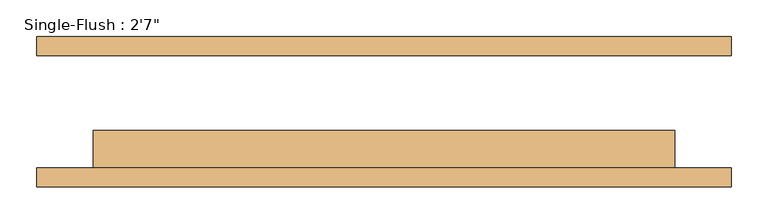
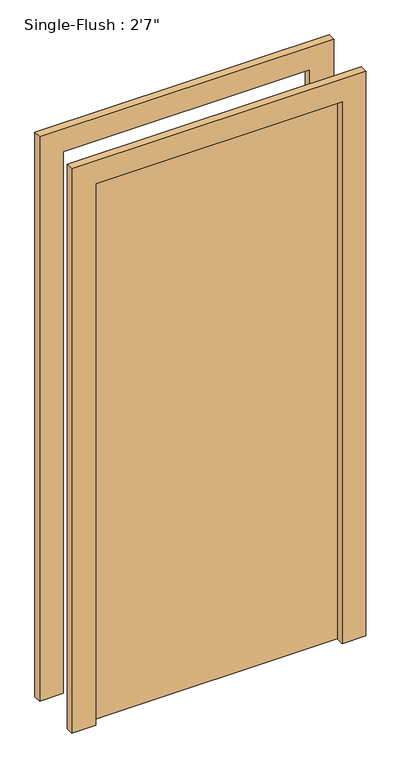
"""IFC4 building model written with IfcOpenShell, lengths in millimetres: door geometry."""

from ifc_helpers import new_model, si_unit, frame, origin, origin_with_axes, place, context, project, spatial, polyline, outline, extrude, source, transform, mapped, element, save


def door_ee35e093(model_context):
    return source(origin(), model_context, "Body", "SweptSolid", [
        extrude(outline(polyline([(1905.0, -469.9), (0.0, -469.9), (0.0, -393.7), (1828.8, -393.7), (1828.8, 393.7), (0.0, 393.7), (0.0, 469.9), (1905.0, 469.9), (1905.0, -469.9)])), frame((0.0, -101.6, 0.0), z_axis=(0.0, 1.0, 0.0), x_axis=(0.0, 0.0, 1.0)), (0.0, 0.0, 1.0), 25.4),
        extrude(outline(polyline([(1905.0, 469.9), (1905.0, -469.9), (0.0, -469.9), (0.0, -393.7), (1828.8, -393.7), (1828.8, 393.7), (0.0, 393.7), (0.0, 469.9), (1905.0, 469.9)])), frame((0.0, 76.2, 0.0), z_axis=(0.0, 1.0, 0.0), x_axis=(0.0, 0.0, 1.0)), (0.0, 0.0, 1.0), 25.4),
        extrude(outline(polyline([(393.7, -25.4), (393.7, -76.2), (-393.7, -76.2), (-393.7, -25.4), (393.7, -25.4)])), origin_with_axes(), (0.0, 0.0, 1.0), 1828.8),
    ])


if __name__ == "__main__":
    model = new_model("IFC4")
    model_context = context("Model", 3, world=origin())
    ifc_project = project(units=[si_unit("LENGTHUNIT", "METRE", prefix="MILLI")], contexts=[model_context])
    site = spatial("IfcSite", under=ifc_project)
    building = spatial("IfcBuilding", under=site)
    placement = place(None, origin())
    door_shape = door_ee35e093(model_context)
    element("IfcDoor", 1, ObjectType="Single-Flush : 2'7\"", at=placement, inside=building, context=model_context, shape_type="MappedRepresentation", body=[
        mapped(door_shape, transform((0.0, 0.0, 0.0), x_axis=(1.0, 0.0, 0.0), y_axis=(0.0, 1.0, 0.0), z_axis=(0.0, 0.0, 1.0))),
    ])
    save(model, "model.ifc")

# Revit data of these elements
# Type "Single-Flush : 2'7\""
#   Type Mark = "12"
#   Construction Type Id = "MDOOR"
#   Assembly Code = "C1020"
#   Analytic Construction = "Metal"
#   Thickness = 0' - 2"
#   Heat Transfer Coefficient (U) = 0.651978 BTU/(h·ft²·°F)
#   Height = 6' - 0"
#   Trim Projection Ext = 0' - 1"
#   Trim Projection Int = 0' - 1"
#   Trim Width = 0' - 3"
#   Width = 2' - 7"
#   Define Thermal Properties by = 1
#   Door Material = Door - Panel
#   Frame Material = Door - Frame
#   Visual Light Transmittance = 0
#   Solar Heat Gain Coefficient = 0
#   Function = (empty or 0)
#   Wall Closure = (empty or 0)
# Element 1 (IfcDoor, "Single-Flush : 2'7\"")
#   Materials on its faces: "Door - Frame", "Door - Panel"
# Materials
#   "Door - Panel": class "Wood", colour RGB 210 159 95, transparency 0, Cost = 0
#   "Door - Frame": colour RGB 118 70 51, transparency 0, Cost = 0
